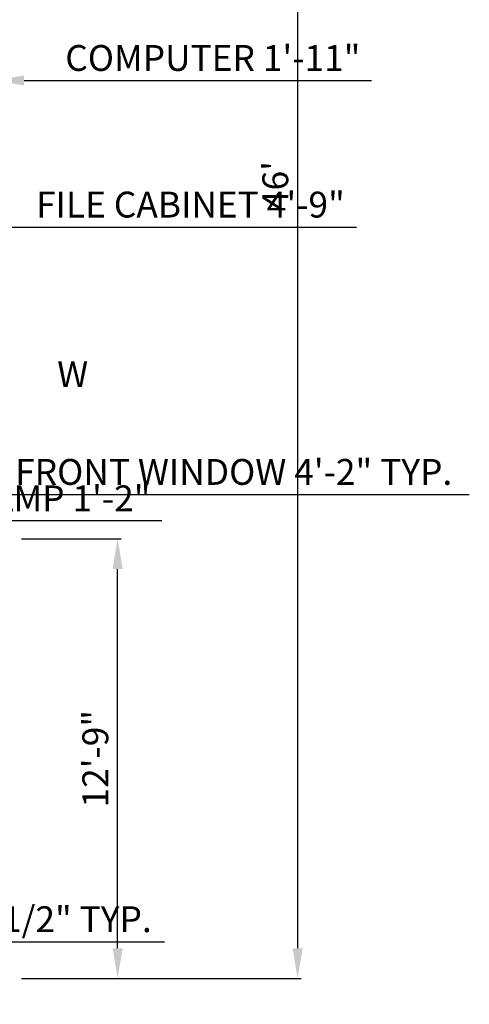
# Model space of a CAD drawing. Units: inches. Extents: x 1956 to 4770, y 1551 to 2596.
# Tile 5 of 10: x 2501 to 2658, y 1748 to 2091. Entities that reach past the tile are written whole.
import ezdxf

# ---------------------------------------------------------------- set-up
doc = ezdxf.new("R2010")
doc.units = ezdxf.units.IN
doc.layers.add('A-ANNO-DIMS', color=2, linetype='Continuous', lineweight=18)
doc.layers.add('A-ANNO-TEXT', color=7, linetype='Continuous', lineweight=18)
doc.styles.get("Standard").update_dxf_attribs({"font": 'arial.ttf'})
doc.dimstyles.new('ISO-25', dxfattribs={"dimtxt": 9, "dimasz": 10.5, "dimexe": 1.25, "dimexo": 0.625, "dimgap": 2, "dimtad": 1, "dimdec": 1, "dimlunit": 4, "dimtxsty": 'Standard', "dimcen": 2.5, "dimadec": 0, "dimazin": 0, "dimtfac": 1, "dimtdec": 1, "dimtmove": 0, "dimatfit": 3, "dimfxl": 1, "dimarcsym": 0})

# ---------------------------------------------------------------- blocks, each defined once
blk = doc.blocks.new('*D1')
at = {"layer": 'A-ANNO-DIMS', "color": 0, "lineweight": -2, "transparency": 16777216}
for p, q in [((2501.88, 2309.09), (2599.11, 2309.09)), ((2597.86, 2298.59), (2597.86, 1767.59)), ((2501.88, 1757.09), (2599.11, 1757.09))]:
    blk.add_line(p, q, dxfattribs=at)
at = {"layer": 'A-ANNO-DIMS', "color": 0, "transparency": 16777216}
for points in [[(2596.11, 2298.59), (2599.61, 2298.59), (2597.86, 2309.09)], [(2596.11, 1767.59), (2599.61, 1767.59), (2597.86, 1757.09)]]:
    blk.add_solid(points, dxfattribs=at)
at = {"layer": 'Defpoints', "color": 0, "transparency": 16777216}
for p in [(2501.25, 2309.09), (2501.25, 1757.09), (2597.86, 1757.09)]:
    blk.add_point(p, dxfattribs=at)
at = {"layer": 'A-ANNO-DIMS', "color": 0, "transparency": 16777216, "insert": (2591.27, 2033.09), "char_height": 9, "attachment_point": 5, "rotation": 90}
blk.add_mtext("46'", dxfattribs=at)
blk = doc.blocks.new('*D29')
at = {"layer": 'A-ANNO-DIMS', "color": 0, "lineweight": -2, "transparency": 16777216}
for p, q in [((2433.25, 1918.71), (2433.25, 1926.84)), ((2483.25, 1918.71), (2483.25, 1926.84)), ((2443.75, 1925.59), (2472.75, 1925.59)), ((2483.25, 1925.59), (2657.56, 1925.59))]:
    blk.add_line(p, q, dxfattribs=at)
at = {"layer": 'A-ANNO-DIMS', "color": 0, "transparency": 16777216}
for points in [[(2443.75, 1927.34), (2443.75, 1923.84), (2433.25, 1925.59)], [(2472.75, 1927.34), (2472.75, 1923.84), (2483.25, 1925.59)]]:
    blk.add_solid(points, dxfattribs=at)
at = {"layer": 'Defpoints', "color": 0, "transparency": 16777216}
for p in [(2483.25, 1925.59), (2433.25, 1918.09), (2483.25, 1918.09)]:
    blk.add_point(p, dxfattribs=at)
at = {"layer": 'A-ANNO-DIMS', "color": 0, "transparency": 16777216, "insert": (2575.65, 1932.24), "char_height": 9, "attachment_point": 5}
blk.add_mtext('FRONT WINDOW 4\'-2" TYP.', dxfattribs=at)
blk = doc.blocks.new('*D39')
at = {"layer": 'A-ANNO-DIMS', "color": 0, "lineweight": -2, "transparency": 16777216}
for p, q in [((2362.8, 1774.88), (2362.8, 1768.65)), ((2400.2, 1774.88), (2400.2, 1768.65)), ((2373.3, 1769.9), (2389.7, 1769.9)), ((2400.2, 1769.9), (2551.56, 1769.9))]:
    blk.add_line(p, q, dxfattribs=at)
at = {"layer": 'A-ANNO-DIMS', "color": 0, "transparency": 16777216}
for points in [[(2373.3, 1771.65), (2373.3, 1768.15), (2362.8, 1769.9)], [(2389.7, 1771.65), (2389.7, 1768.15), (2400.2, 1769.9)]]:
    blk.add_solid(points, dxfattribs=at)
at = {"layer": 'Defpoints', "color": 0, "transparency": 16777216}
for p in [(2362.8, 1775.51), (2400.2, 1775.51), (2400.2, 1769.9)]:
    blk.add_point(p, dxfattribs=at)
at = {"layer": 'A-ANNO-DIMS', "color": 0, "transparency": 16777216, "insert": (2481.13, 1776.56), "char_height": 9, "attachment_point": 5}
blk.add_mtext('PLANTER 3\'-1 1/2" TYP.', dxfattribs=at)
blk = doc.blocks.new('*D47')
at = {"layer": 'A-ANNO-DIMS', "color": 0, "lineweight": -2, "transparency": 16777216}
for p, q in [((2395.97, 1916.52), (2385.47, 1916.52)), ((2406.47, 1918), (2406.47, 1915.27)), ((2406.47, 1916.52), (2420.47, 1916.52)), ((2420.47, 1918), (2420.47, 1915.27)), ((2430.97, 1916.52), (2550.67, 1916.52))]:
    blk.add_line(p, q, dxfattribs=at)
at = {"layer": 'A-ANNO-DIMS', "color": 0, "transparency": 16777216}
for points in [[(2395.97, 1918.27), (2395.97, 1914.77), (2406.47, 1916.52)], [(2430.97, 1918.27), (2430.97, 1914.77), (2420.47, 1916.52)]]:
    blk.add_solid(points, dxfattribs=at)
at = {"layer": 'Defpoints', "color": 0, "transparency": 16777216}
for p in [(2406.47, 1918.62), (2420.47, 1918.62), (2420.47, 1916.52)]:
    blk.add_point(p, dxfattribs=at)
at = {"layer": 'A-ANNO-DIMS', "color": 0, "transparency": 16777216, "insert": (2496.07, 1923.04), "char_height": 9, "attachment_point": 5}
blk.add_mtext('TABLE LAMP 1\'-2"', dxfattribs=at)
blk = doc.blocks.new('*D53')
at = {"layer": 'A-ANNO-DIMS', "color": 0, "lineweight": -2, "transparency": 16777216}
for p, q in [((2469.27, 2066.83), (2469.27, 2070.91)), ((2492.27, 2066.83), (2492.27, 2070.91)), ((2458.77, 2069.66), (2448.27, 2069.66)), ((2469.27, 2069.66), (2492.27, 2069.66)), ((2502.77, 2069.66), (2623.52, 2069.66))]:
    blk.add_line(p, q, dxfattribs=at)
at = {"layer": 'A-ANNO-DIMS', "color": 0, "transparency": 16777216}
for points in [[(2458.77, 2071.41), (2458.77, 2067.91), (2469.27, 2069.66)], [(2502.77, 2071.41), (2502.77, 2067.91), (2492.27, 2069.66)]]:
    blk.add_solid(points, dxfattribs=at)
at = {"layer": 'Defpoints', "color": 0, "transparency": 16777216}
for p in [(2492.27, 2069.66), (2469.27, 2066.21), (2492.27, 2066.21)]:
    blk.add_point(p, dxfattribs=at)
at = {"layer": 'A-ANNO-DIMS', "color": 0, "transparency": 16777216, "insert": (2568.4, 2076.31), "char_height": 9, "attachment_point": 5}
blk.add_mtext('COMPUTER 1\'-11"', dxfattribs=at)
blk = doc.blocks.new('*D55')
at = {"layer": 'A-ANNO-DIMS', "color": 0, "lineweight": -2, "transparency": 16777216}
for p, q in [((2435.39, 2026.56), (2435.39, 2017.38)), ((2492.39, 2026.56), (2492.39, 2017.38)), ((2445.89, 2018.63), (2481.89, 2018.63)), ((2492.39, 2018.63), (2618.34, 2018.63))]:
    blk.add_line(p, q, dxfattribs=at)
at = {"layer": 'A-ANNO-DIMS', "color": 0, "transparency": 16777216}
for points in [[(2445.89, 2020.38), (2445.89, 2016.88), (2435.39, 2018.63)], [(2481.89, 2020.38), (2481.89, 2016.88), (2492.39, 2018.63)]]:
    blk.add_solid(points, dxfattribs=at)
at = {"layer": 'Defpoints', "color": 0, "transparency": 16777216}
for p in [(2435.39, 2027.18), (2492.39, 2027.18), (2492.39, 2018.63)]:
    blk.add_point(p, dxfattribs=at)
at = {"layer": 'A-ANNO-DIMS', "color": 0, "transparency": 16777216, "insert": (2560.61, 2025.28), "char_height": 9, "attachment_point": 5}
blk.add_mtext('FILE CABINET 4\'-9"', dxfattribs=at)
blk = doc.blocks.new('*D64')
at = {"layer": 'A-ANNO-DIMS', "color": 0, "lineweight": -2, "transparency": 16777216}
for p, q in [((2501.88, 1910.09), (2536.55, 1910.09)), ((2535.3, 1767.59), (2535.3, 1899.59)), ((2501.88, 1757.09), (2536.55, 1757.09))]:
    blk.add_line(p, q, dxfattribs=at)
at = {"layer": 'A-ANNO-DIMS', "color": 0, "transparency": 16777216}
for points in [[(2533.55, 1899.59), (2537.05, 1899.59), (2535.3, 1910.09)], [(2533.55, 1767.59), (2537.05, 1767.59), (2535.3, 1757.09)]]:
    blk.add_solid(points, dxfattribs=at)
at = {"layer": 'Defpoints', "color": 0, "transparency": 16777216}
for p in [(2501.25, 1910.09), (2535.3, 1910.09), (2501.25, 1757.09)]:
    blk.add_point(p, dxfattribs=at)
at = {"layer": 'A-ANNO-DIMS', "color": 0, "transparency": 16777216, "insert": (2528.71, 1833.59), "char_height": 9, "attachment_point": 5, "rotation": 90}
blk.add_mtext('12\'-9"', dxfattribs=at)

msp = doc.modelspace()

# ---------------------------------------------------------------- texts
at = {"layer": 'A-ANNO-TEXT'}
msp.add_text('W', height=9, dxfattribs=at).set_placement((2514.28, 1962.93))

# ---------------------------------------------------------------- dimensions: what is measured, and where the dimension line sits
at = {"layer": 'A-ANNO-DIMS'}
for base, p1, p2, override, picture, middle in [((2597.86, 1757.09), (2501.25, 2309.09), (2501.25, 1757.09), {"dimclrd": 0, "dimclre": 0, "dimclrt": 0}, '*D1', (2591.27, 2033.09)), ((2535.3, 1910.09), (2501.25, 1757.09), (2501.25, 1910.09), {"dimdec": 1, "dimlfac": 1, "dimrnd": 0, "dimzin": 1, "dimdsep": 46, "dimlunit": 4, "dimfrac": 2}, '*D64', (2528.71, 1833.59))]:
    dim = msp.add_linear_dim(base=base, p1=p1, p2=p2, angle=90, dimstyle='ISO-25', override=override, dxfattribs=at)
    dim.commit()
    dim.dimension.update_dxf_attribs({"geometry": picture, "text_midpoint": middle})
for base, p1, p2, text, picture, middle in [((2492.27, 2069.66), (2469.27, 2066.21), (2492.27, 2066.21), 'COMPUTER <>', '*D53', (2568.4, 2076.31)), ((2492.39, 2018.63), (2435.39, 2027.18), (2492.39, 2027.18), 'FILE CABINET <>', '*D55', (2560.61, 2025.28)), ((2483.25, 1925.59), (2433.25, 1918.09), (2483.25, 1918.09), 'FRONT WINDOW <> TYP.', '*D29', (2575.65, 1932.24)), ((2420.47, 1916.52), (2406.47, 1918.62), (2420.47, 1918.62), 'TABLE LAMP <>', '*D47', (2496.07, 1923.04)), ((2400.2, 1769.9), (2362.8, 1775.51), (2400.2, 1775.51), 'PLANTER <> TYP.', '*D39', (2481.13, 1776.56))]:
    dim = msp.add_linear_dim(base=base, p1=p1, p2=p2, text=text, dimstyle='ISO-25', override={"dimdec": 1, "dimlfac": 1, "dimrnd": 0, "dimzin": 1, "dimdsep": 46, "dimlunit": 4, "dimfrac": 2}, dxfattribs=at)
    dim.commit()
    dim.dimension.update_dxf_attribs({"geometry": picture, "text_midpoint": middle})

doc.saveas('drawing.dxf')
